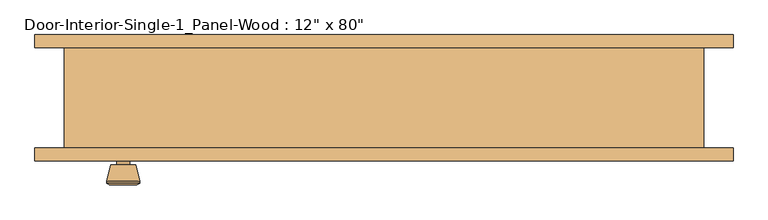
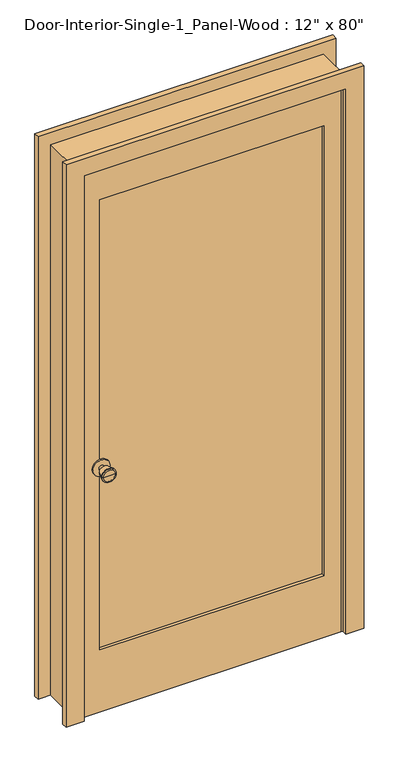
"""IFC4 building model written with IfcOpenShell, lengths in millimetres: door geometry."""

from ifc_helpers import new_model, si_unit, point, frame, frame_2d, origin, place, context, project, spatial, polyline, circle_curve, trimmed, segment, composite_curve, outline, extrude, faceted_brep, source, transform, mapped, element, save
from ifc_brep_helpers import plane_surface, cylinder_surface, revolved_surface, advanced_brep


def door_792ab218(model_context):
    return source(origin(), model_context, "Body", "SolidModel", [
        advanced_brep(
        [(-393.7, -32.1, 914.4), (-403.7, -32.1, 914.4), (-383.7, -32.1, 914.4), (-373.2241324, 16.9, 914.4), (-414.1758676, 16.9, 914.4), (-393.7, 16.9, 914.4), (-368.7, 15.0721319, 914.4), (-418.7, 15.0721319, 914.4), (-368.7, 11.6084537, 914.4), (-418.7, 11.6084537, 914.4), (-375.063764, -13.1, 914.4), (-412.336236, -13.1, 914.4), (-383.7, -13.1, 914.4), (-403.7, -13.1, 914.4)],
        [
            (0, 1),
            (1, 2, circle_curve(frame((-393.7, -32.1, 914.4), z_axis=(0.0, -1.0, 0.0), x_axis=(-1.0, 0.0, 0.0)), 10.0)),
            (2, 0),
            (2, 1, circle_curve(frame((-393.7, -32.1, 914.4), z_axis=(0.0, -1.0, 0.0), x_axis=(-1.0, 0.0, 0.0)), 10.0)),
            (3, 4, circle_curve(frame((-393.7, 16.9, 914.4), z_axis=(0.0, 1.0, 0.0), x_axis=(-1.0, 0.0, 0.0)), 20.4758676)),
            (4, 5),
            (5, 3),
            (4, 3, circle_curve(frame((-393.7, 16.9, 914.4), z_axis=(0.0, 1.0, 0.0), x_axis=(-1.0, 0.0, 0.0)), 20.4758676)),
            (6, 7, circle_curve(frame((-393.7, 15.0721319, 914.4), z_axis=(0.0, 1.0, 0.0), x_axis=(-1.0, 0.0, 0.0)), 25.0)),
            (7, 4),
            (3, 6),
            (7, 6, circle_curve(frame((-393.7, 15.0721319, 914.4), z_axis=(0.0, 1.0, 0.0), x_axis=(-1.0, 0.0, 0.0)), 25.0)),
            (8, 9, circle_curve(frame((-393.7, 11.6084537, 914.4), z_axis=(0.0, 1.0, 0.0), x_axis=(-1.0, 0.0, 0.0)), 25.0)),
            (9, 7),
            (6, 8),
            (9, 8, circle_curve(frame((-393.7, 11.6084537, 914.4), z_axis=(0.0, 1.0, 0.0), x_axis=(-1.0, 0.0, 0.0)), 25.0)),
            (10, 11, circle_curve(frame((-393.7, -13.1, 914.4), z_axis=(0.0, 1.0, 0.0), x_axis=(-1.0, 0.0, 0.0)), 18.636236)),
            (11, 9),
            (8, 10),
            (11, 10, circle_curve(frame((-393.7, -13.1, 914.4), z_axis=(0.0, 1.0, 0.0), x_axis=(-1.0, 0.0, 0.0)), 18.636236)),
            (12, 13, circle_curve(frame((-393.7, -13.1, 914.4), z_axis=(0.0, 1.0, 0.0), x_axis=(-1.0, 0.0, 0.0)), 10.0)),
            (13, 11),
            (10, 12),
            (13, 12, circle_curve(frame((-393.7, -13.1, 914.4), z_axis=(0.0, 1.0, 0.0), x_axis=(-1.0, 0.0, 0.0)), 10.0)),
            (1, 13),
            (12, 2),
        ],
        [
            plane_surface(frame((-393.7, -32.1, 914.4), z_axis=(0.0, -1.0, 0.0), x_axis=(-1.0, 0.0, 0.0))),
            plane_surface(frame((-393.7, 16.9, 914.4), z_axis=(0.0, 1.0, 0.0), x_axis=(-1.0, 0.0, 0.0))),
            revolved_surface(polyline([(-414.1758676, 16.9, 914.4), (-418.7, 15.0721319, 914.4)]), (-393.7, -32.1, 914.4), (0.0, -1.0, 0.0)),
            cylinder_surface(frame((-393.7, -32.1, 914.4), z_axis=(0.0, -1.0, 0.0), x_axis=(-1.0, 0.0, 0.0)), 25.0),
            revolved_surface(polyline([(-418.7, 11.6084537, 914.4), (-412.336236, -13.1, 914.4)]), (-393.7, -32.1, 914.4), (0.0, -1.0, 0.0)),
            plane_surface(frame((-393.7, -13.1, 914.4), z_axis=(0.0, -1.0, 0.0), x_axis=(-1.0, 0.0, 0.0))),
            cylinder_surface(frame((-393.7, -32.1, 914.4), z_axis=(0.0, -1.0, 0.0), x_axis=(-1.0, 0.0, 0.0)), 10.0),
        ],
        [
            (0, [[1, 2, 3]]),
            (0, [[-3, 4, -1]]),
            (1, [[5, 6, 7]]),
            (1, [[8, -7, -6]]),
            (2, [[9, 10, -5, 11]]),
            (2, [[12, -11, -8, -10]]),
            (3, [[13, 14, -9, 15]]),
            (3, [[16, -15, -12, -14]]),
            (4, [[17, 18, -13, 19]]),
            (4, [[20, -19, -16, -18]]),
            (5, [[21, 22, -17, 23]]),
            (5, [[24, -23, -20, -22]]),
            (6, [[-2, 25, -21, 26]]),
            (6, [[-4, -26, -24, -25]]),
        ],
    ),
        extrude(outline(composite_curve([segment(trimmed(circle_curve(frame_2d((914.4, -393.7)), 30.0), [point((914.4, -423.7))], [point((914.4, -363.7))], False, "CARTESIAN"), True, "CONTINUOUS"), segment(trimmed(circle_curve(frame_2d((914.4, -393.7)), 30.0), [point((914.4, -363.7))], [point((914.4, -423.7))], False, "CARTESIAN"), True, "CONTINUOUS")], self_intersect=False)), frame((0.0, -38.1, 0.0), z_axis=(0.0, 1.0, 0.0), x_axis=(0.0, 0.0, 1.0)), (0.0, 0.0, 1.0), 6.0),
        advanced_brep(
        [(-393.7, -79.025, 914.4), (-383.7, -79.025, 914.4), (-403.7, -79.025, 914.4), (-373.2241324, -128.025, 914.4), (-393.7, -128.025, 914.4), (-414.1758676, -128.025, 914.4), (-368.7, -126.1971319, 914.4), (-418.7, -126.1971319, 914.4), (-368.7, -122.7334537, 914.4), (-418.7, -122.7334537, 914.4), (-375.063764, -98.025, 914.4), (-412.336236, -98.025, 914.4), (-383.7, -98.025, 914.4), (-403.7, -98.025, 914.4)],
        [
            (0, 1),
            (1, 2, circle_curve(frame((-393.7, -79.025, 914.4), z_axis=(0.0, 1.0, 0.0), x_axis=(-1.0, 0.0, 0.0)), 10.0)),
            (2, 0),
            (2, 1, circle_curve(frame((-393.7, -79.025, 914.4), z_axis=(0.0, 1.0, 0.0), x_axis=(-1.0, 0.0, 0.0)), 10.0)),
            (3, 4),
            (4, 5),
            (5, 3, circle_curve(frame((-393.7, -128.025, 914.4), z_axis=(0.0, -1.0, 0.0), x_axis=(-1.0, 0.0, 0.0)), 20.4758676)),
            (3, 5, circle_curve(frame((-393.7, -128.025, 914.4), z_axis=(0.0, -1.0, 0.0), x_axis=(-1.0, 0.0, 0.0)), 20.4758676)),
            (6, 3),
            (5, 7),
            (7, 6, circle_curve(frame((-393.7, -126.1971319, 914.4), z_axis=(0.0, -1.0, 0.0), x_axis=(-1.0, 0.0, 0.0)), 25.0)),
            (6, 7, circle_curve(frame((-393.7, -126.1971319, 914.4), z_axis=(0.0, -1.0, 0.0), x_axis=(-1.0, 0.0, 0.0)), 25.0)),
            (8, 6),
            (7, 9),
            (9, 8, circle_curve(frame((-393.7, -122.7334537, 914.4), z_axis=(0.0, -1.0, 0.0), x_axis=(-1.0, 0.0, 0.0)), 25.0)),
            (8, 9, circle_curve(frame((-393.7, -122.7334537, 914.4), z_axis=(0.0, -1.0, 0.0), x_axis=(-1.0, 0.0, 0.0)), 25.0)),
            (10, 8),
            (9, 11),
            (11, 10, circle_curve(frame((-393.7, -98.025, 914.4), z_axis=(0.0, -1.0, 0.0), x_axis=(-1.0, 0.0, 0.0)), 18.636236)),
            (10, 11, circle_curve(frame((-393.7, -98.025, 914.4), z_axis=(0.0, -1.0, 0.0), x_axis=(-1.0, 0.0, 0.0)), 18.636236)),
            (12, 10),
            (11, 13),
            (13, 12, circle_curve(frame((-393.7, -98.025, 914.4), z_axis=(0.0, -1.0, 0.0), x_axis=(-1.0, 0.0, 0.0)), 10.0)),
            (12, 13, circle_curve(frame((-393.7, -98.025, 914.4), z_axis=(0.0, -1.0, 0.0), x_axis=(-1.0, 0.0, 0.0)), 10.0)),
            (1, 12),
            (13, 2),
        ],
        [
            plane_surface(frame((-393.7, -79.025, 914.4), z_axis=(0.0, 1.0, 0.0), x_axis=(-1.0, 0.0, 0.0))),
            plane_surface(frame((-393.7, -128.025, 914.4), z_axis=(0.0, -1.0, 0.0), x_axis=(-1.0, 0.0, 0.0))),
            revolved_surface(polyline([(-414.1758676, -128.025, 914.4), (-418.7, -126.1971319, 914.4)]), (-393.7, -79.025, 914.4), (0.0, 1.0, 0.0)),
            cylinder_surface(frame((-393.7, -79.025, 914.4), z_axis=(0.0, 1.0, 0.0), x_axis=(-1.0, 0.0, 0.0)), 25.0),
            revolved_surface(polyline([(-418.7, -122.7334537, 914.4), (-412.336236, -98.025, 914.4)]), (-393.7, -79.025, 914.4), (0.0, 1.0, 0.0)),
            plane_surface(frame((-393.7, -98.025, 914.4), z_axis=(0.0, 1.0, 0.0), x_axis=(-1.0, 0.0, 0.0))),
            cylinder_surface(frame((-393.7, -79.025, 914.4), z_axis=(0.0, 1.0, 0.0), x_axis=(-1.0, 0.0, 0.0)), 10.0),
        ],
        [
            (0, [[1, 2, 3]]),
            (0, [[-3, 4, -1]]),
            (1, [[5, 6, 7]]),
            (1, [[-6, -5, 8]]),
            (2, [[9, -7, 10, 11]]),
            (2, [[-10, -8, -9, 12]]),
            (3, [[13, -11, 14, 15]]),
            (3, [[-14, -12, -13, 16]]),
            (4, [[17, -15, 18, 19]]),
            (4, [[-18, -16, -17, 20]]),
            (5, [[21, -19, 22, 23]]),
            (5, [[-22, -20, -21, 24]]),
            (6, [[25, -23, 26, -2]]),
            (6, [[-26, -24, -25, -4]]),
        ],
    ),
        extrude(outline(composite_curve([segment(trimmed(circle_curve(frame_2d((914.4, -393.7)), 30.0), [point((914.4, -423.7))], [point((914.4, -363.7))], False, "CARTESIAN"), True, "CONTINUOUS"), segment(trimmed(circle_curve(frame_2d((914.4, -393.7)), 30.0), [point((914.4, -363.7))], [point((914.4, -423.7))], False, "CARTESIAN"), True, "CONTINUOUS")], self_intersect=False)), frame((0.0, -79.025, 0.0), z_axis=(0.0, 1.0, 0.0), x_axis=(0.0, 0.0, 1.0)), (0.0, 0.0, 1.0), 6.0),
        extrude(outline(polyline([(396.875, -49.7416667), (396.875, -61.3833333), (-396.875, -61.3833333), (-396.875, -49.7416667), (396.875, -49.7416667)])), frame((0.0, 0.0, 231.775), z_axis=(0.0, 0.0, 1.0), x_axis=(1.0, 0.0, 0.0)), (0.0, 0.0, 1.0), 1681.1625),
        extrude(outline(polyline([(2032.0, -457.2), (0.0, -457.2), (0.0, 457.2), (2032.0, 457.2), (2032.0, -457.2)]), holes=[polyline([(1912.9375, -396.875), (1912.9375, 396.875), (231.775, 396.875), (231.775, -396.875), (1912.9375, -396.875)])]), frame((0.0, -73.025, 0.0), z_axis=(0.0, 1.0, 0.0), x_axis=(0.0, 0.0, 1.0)), (0.0, 0.0, 1.0), 34.925),
        faceted_brep([(482.6, -73.025, 0.0), (457.2, -73.025, 0.0), (457.2, -38.1, 0.0), (444.5, -38.1, 0.0), (444.5, -3.175, 0.0), (457.2, -3.175, 0.0), (457.2, 79.375, 0.0), (482.6, 79.375, 0.0), (482.6, 79.375, 2057.4), (482.6, -73.025, 2057.4), (457.2, 79.375, 2032.0), (-457.2, 79.375, 2032.0), (-457.2, 79.375, 0.0), (-482.6, 79.375, 0.0), (-482.6, 79.375, 2057.4), (457.2, -3.175, 2032.0), (444.5, -3.175, 2019.3), (-444.5, -3.175, 2019.3), (-444.5, -3.175, 0.0), (-457.2, -3.175, 0.0), (-457.2, -3.175, 2032.0), (444.5, -38.1, 2019.3), (457.2, -38.1, 2032.0), (-457.2, -38.1, 2032.0), (-457.2, -38.1, 0.0), (-444.5, -38.1, 0.0), (-444.5, -38.1, 2019.3), (457.2, -73.025, 2032.0), (-482.6, -73.025, 2057.4), (-482.6, -73.025, 0.0), (-457.2, -73.025, 0.0), (-457.2, -73.025, 2032.0)], [[[0, 1, 2, 3, 4, 5, 6, 7]], [[7, 8, 9, 0]], [[6, 10, 11, 12, 13, 14, 8, 7]], [[5, 15, 10, 6]], [[4, 16, 17, 18, 19, 20, 15, 5]], [[3, 21, 16, 4]], [[2, 22, 23, 24, 25, 26, 21, 3]], [[1, 27, 22, 2]], [[0, 9, 28, 29, 30, 31, 27, 1]], [[8, 14, 28, 9]], [[15, 20, 11, 10]], [[21, 26, 17, 16]], [[27, 31, 23, 22]], [[29, 13, 12, 19, 18, 25, 24, 30]], [[14, 13, 29, 28]], [[20, 19, 12, 11]], [[26, 25, 18, 17]], [[31, 30, 24, 23]]]),
        extrude(outline(polyline([(0.0, 527.05), (2101.85, 527.05), (2101.85, -527.05), (0.0, -527.05), (0.0, -463.55), (2038.35, -463.55), (2038.35, 463.55), (0.0, 463.55), (0.0, 527.05)])), frame((0.0, 79.375, 0.0), z_axis=(0.0, 1.0, 0.0), x_axis=(0.0, 0.0, 1.0)), (0.0, 0.0, 1.0), 19.05),
        extrude(outline(polyline([(0.0, 527.05), (2101.85, 527.05), (2101.85, -527.05), (0.0, -527.05), (0.0, -463.55), (2038.35, -463.55), (2038.35, 463.55), (0.0, 463.55), (0.0, 527.05)])), frame((0.0, -92.075, 0.0), z_axis=(0.0, 1.0, 0.0), x_axis=(0.0, 0.0, 1.0)), (0.0, 0.0, 1.0), 19.05),
    ])


if __name__ == "__main__":
    model = new_model("IFC4")
    model_context = context("Model", 3, world=origin())
    ifc_project = project(units=[si_unit("LENGTHUNIT", "METRE", prefix="MILLI")], contexts=[model_context])
    site = spatial("IfcSite", under=ifc_project)
    building = spatial("IfcBuilding", under=site)
    placement = place(None, origin())
    door_shape = door_792ab218(model_context)
    element("IfcDoor", 1, ObjectType="Door-Interior-Single-1_Panel-Wood : 12\" x 80\"", at=placement, inside=building, context=model_context, shape_type="MappedRepresentation", body=[
        mapped(door_shape, transform((0.0, 0.0, 0.0), x_axis=(1.0, 0.0, 0.0), y_axis=(0.0, 1.0, 0.0), z_axis=(0.0, 0.0, 1.0))),
    ])
    save(model, "model.ifc")

# Revit data of these elements
# Type "Door-Interior-Single-1_Panel-Wood : 12\" x 80\""
#   Type Mark = "9"
#   Assembly Code = "C1020300"
#   Analytic Construction = "Wooden"
#   Top Rail = 0' - 4 11/16"
#   Thickness = 0' - 1 3/8"
#   Thermal Resistance (R) = 2.5876 (h·ft²·°F)/BTU
#   Swing Angle [instance default] = 90.00°
#   Stiles = 0' - 2 3/8"
#   Rough Width = 3' - 2"
#   Rough Height = 6' - 9"
#   Height = 6' - 8"
#   Width = 3' - 0"
#   Heat Transfer Coefficient (U) = 0.3865 BTU/(h·ft²·°F)
#   Bottom Rail = 0' - 9 1/8"
#   Trim Material = Cherry
#   Panel Material = Cherry
#   Frame Material = Cherry
#   Door Handle Material = Aluminum
#   Visual Light Transmittance = 0
#   Solar Heat Gain Coefficient = 0
#   Wall Closure = (empty or 0)
#   Function = (empty or 0)
# Element 1 (IfcDoor, "Door-Interior-Single-1_Panel-Wood : 12\" x 80\"")
#   Materials on its faces: "Cherry", "Aluminum"
# Materials
#   "Cherry": class "Wood", colour RGB 226 177 128, transparency 0, Description = "Prunus Serotina", Cost = 0
#   "Aluminum": class "Metal", colour RGB 247 247 247, transparency 0, Description = "Aluminum 6061", Cost = 0
